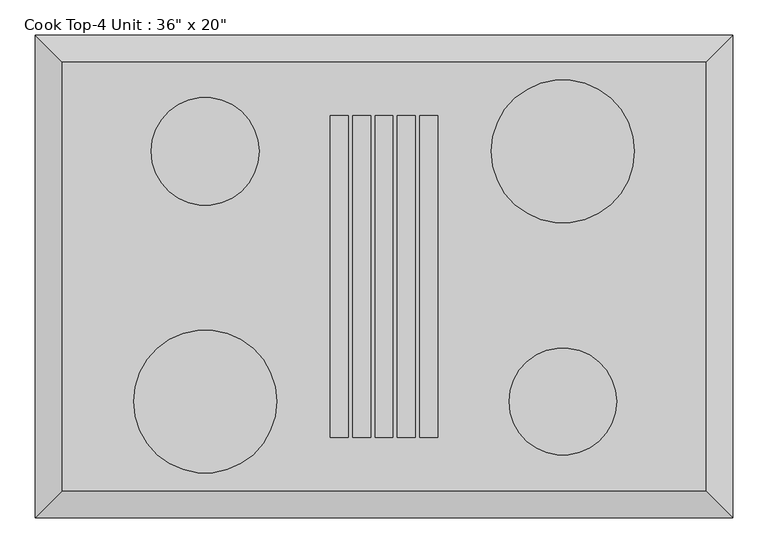
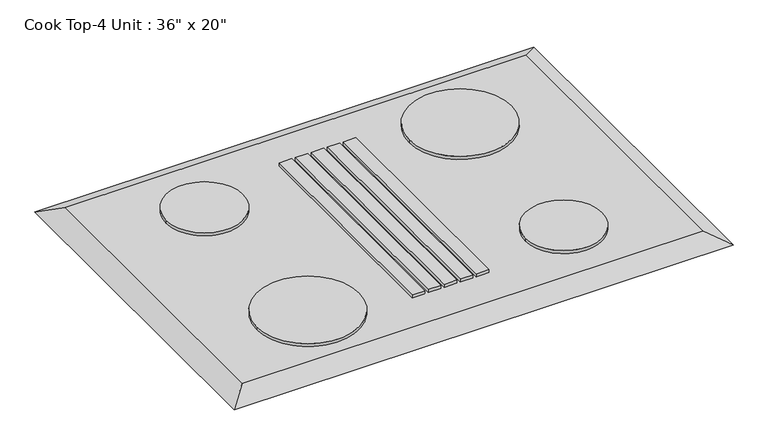
"""IFC4 building model written with IfcOpenShell, lengths in millimetres: proxy geometry."""

from ifc_helpers import new_model, si_unit, point, frame, frame_2d, origin, place, context, project, spatial, polyline, circle_curve, trimmed, segment, composite_curve, outline, extrude, faceted_brep, source, transform, mapped, element, save


def proxy_bb1e6e30(model_context):
    return source(origin(), model_context, "Body", "SolidModel", [
        extrude(outline(composite_curve([segment(trimmed(circle_curve(frame_2d((-254.0, 177.8)), 76.5869489), [point((-177.4130511, 177.8))], [point((-330.5869489, 177.8))], False, "CARTESIAN"), True, "CONTINUOUS"), segment(trimmed(circle_curve(frame_2d((-254.0, 177.8)), 76.5869489), [point((-330.5869489, 177.8))], [point((-177.4130511, 177.8))], False, "CARTESIAN"), True, "CONTINUOUS")], self_intersect=False)), frame((0.0, 0.0, 806.45), z_axis=(0.0, 0.0, 1.0), x_axis=(1.0, 0.0, 0.0)), (0.0, 0.0, 1.0), 6.35),
        extrude(outline(composite_curve([segment(trimmed(circle_curve(frame_2d((254.0, 177.8)), 101.6), [point((355.6, 177.8))], [point((152.4, 177.8))], False, "CARTESIAN"), True, "CONTINUOUS"), segment(trimmed(circle_curve(frame_2d((254.0, 177.8)), 101.6), [point((152.4, 177.8))], [point((355.6, 177.8))], False, "CARTESIAN"), True, "CONTINUOUS")], self_intersect=False)), frame((0.0, 0.0, 806.45), z_axis=(0.0, 0.0, 1.0), x_axis=(1.0, 0.0, 0.0)), (0.0, 0.0, 1.0), 6.35),
        extrude(outline(composite_curve([segment(trimmed(circle_curve(frame_2d((254.0, -177.8)), 76.2), [point((330.2, -177.8))], [point((177.8, -177.8))], False, "CARTESIAN"), True, "CONTINUOUS"), segment(trimmed(circle_curve(frame_2d((254.0, -177.8)), 76.2), [point((177.8, -177.8))], [point((330.2, -177.8))], False, "CARTESIAN"), True, "CONTINUOUS")], self_intersect=False)), frame((0.0, 0.0, 806.45), z_axis=(0.0, 0.0, 1.0), x_axis=(1.0, 0.0, 0.0)), (0.0, 0.0, 1.0), 6.35),
        extrude(outline(polyline([(-50.8, 228.6), (-50.8, -228.6), (-76.2, -228.6), (-76.2, 228.6), (-50.8, 228.6)])), frame((0.0, 0.0, 806.45), z_axis=(0.0, 0.0, 1.0), x_axis=(1.0, 0.0, 0.0)), (0.0, 0.0, 1.0), 6.35),
        extrude(outline(polyline([(-19.05, 228.6), (-19.05, -228.6), (-44.45, -228.6), (-44.45, 228.6), (-19.05, 228.6)])), frame((0.0, 0.0, 806.45), z_axis=(0.0, 0.0, 1.0), x_axis=(1.0, 0.0, 0.0)), (0.0, 0.0, 1.0), 6.35),
        extrude(outline(polyline([(12.7, 228.6), (12.7, -228.6), (-12.7, -228.6), (-12.7, 228.6), (12.7, 228.6)])), frame((0.0, 0.0, 806.45), z_axis=(0.0, 0.0, 1.0), x_axis=(1.0, 0.0, 0.0)), (0.0, 0.0, 1.0), 6.35),
        extrude(outline(polyline([(44.45, 228.6), (44.45, -228.6), (19.05, -228.6), (19.05, 228.6), (44.45, 228.6)])), frame((0.0, 0.0, 806.45), z_axis=(0.0, 0.0, 1.0), x_axis=(1.0, 0.0, 0.0)), (0.0, 0.0, 1.0), 6.35),
        extrude(outline(polyline([(76.2, 228.6), (76.2, -228.6), (50.8, -228.6), (50.8, 228.6), (76.2, 228.6)])), frame((0.0, 0.0, 806.45), z_axis=(0.0, 0.0, 1.0), x_axis=(1.0, 0.0, 0.0)), (0.0, 0.0, 1.0), 6.35),
        faceted_brep([(457.2, 304.8, 806.45), (-457.2, 304.8, 806.45), (-457.2, -304.8, 806.45), (457.2, -304.8, 806.45), (495.3, 342.9, 787.4), (495.3, -342.9, 787.4), (-495.3, -342.9, 787.4), (-495.3, 342.9, 787.4)], [[[0, 1, 2, 3]], [[4, 5, 6, 7]], [[4, 7, 1, 0]], [[7, 6, 2, 1]], [[6, 5, 3, 2]], [[5, 4, 0, 3]]]),
        extrude(outline(composite_curve([segment(trimmed(circle_curve(frame_2d((-254.0, -177.8)), 101.6), [point((-152.4, -177.8))], [point((-355.6, -177.8))], False, "CARTESIAN"), True, "CONTINUOUS"), segment(trimmed(circle_curve(frame_2d((-254.0, -177.8)), 101.6), [point((-355.6, -177.8))], [point((-152.4, -177.8))], False, "CARTESIAN"), True, "CONTINUOUS")], self_intersect=False)), frame((0.0, 0.0, 806.45), z_axis=(0.0, 0.0, 1.0), x_axis=(1.0, 0.0, 0.0)), (0.0, 0.0, 1.0), 6.35),
    ])


if __name__ == "__main__":
    model = new_model("IFC4")
    model_context = context("Model", 3, world=origin())
    ifc_project = project(units=[si_unit("LENGTHUNIT", "METRE", prefix="MILLI")], contexts=[model_context])
    site = spatial("IfcSite", under=ifc_project)
    building = spatial("IfcBuilding", under=site)
    placement = place(None, origin())
    proxy_shape = proxy_bb1e6e30(model_context)
    element("IfcBuildingElementProxy", 1, Name="Cook Top-4 Unit : 36\" x 20\"", ObjectType="Cook Top-4 Unit : 36\" x 20\"", at=placement, inside=building, context=model_context, shape_type="MappedRepresentation", body=[
        mapped(proxy_shape, transform((0.0, 0.0, 0.0), x_axis=(1.0, 0.0, 0.0), y_axis=(0.0, 1.0, 0.0), z_axis=(0.0, 0.0, 1.0))),
    ])
    save(model, "model.ifc")

# Revit data of these elements
# Type "Cook Top-4 Unit : 36\" x 20\""
#   Assembly Code = "E1090400"
#   Depth = 2' - 0"
#   Width = 3' - 0"
#   Burner Material = Steel, Chrome Plated
#   Cooktop Material = Steel, Polished
#   Default Elevation = 0
# Element 1 (IfcBuildingElementProxy, "Cook Top-4 Unit : 36\" x 20\"")
#   Materials on its faces: "Steel, Chrome Plated", "Steel, Polished"
# Materials
#   "Steel, Chrome Plated": class "Metal", colour RGB 17 17 17, transparency 0, Description = "Chromiuim plated steel", Cost = 0
#   "Steel, Polished": class "Metal", colour RGB 192 192 192, transparency 0, Description = "Polished steel", Cost = 0
